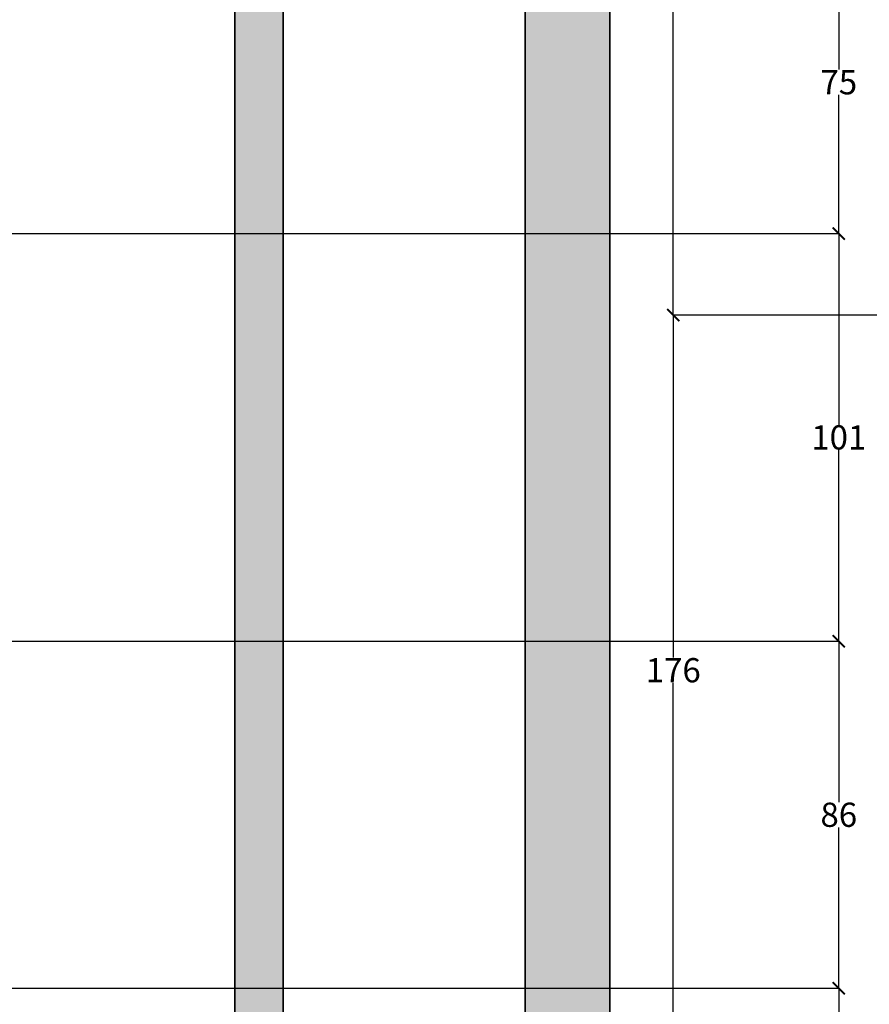
# Model space of a CAD drawing. Units: inches. Extents: x 925 to 2834, y 111 to 1355.
# Tile 12 of 25: x 1785 to 1996, y 638 to 882. Entities that reach past the tile are written whole.
import ezdxf

# ---------------------------------------------------------------- set-up
doc = ezdxf.new("R2010")
doc.units = ezdxf.units.IN
doc.header["$MEASUREMENT"] = 0
for name, color, linetype, lineweight in [('A-ANNO-DIMS', 2, 'Continuous', 18), ('A-ANNO-TTLB', 7, 'Continuous', 35), ('A-FLOR-PATT', 252, 'Continuous', 13)]:
    doc.layers.add(name, color=color, linetype=linetype, lineweight=lineweight)
doc.styles.get("Standard").update_dxf_attribs({"font": 'arial.ttf'})
doc.dimstyles.get("Standard").update_dxf_attribs({"dimtxt": 6, "dimasz": 3, "dimexe": 0.18, "dimexo": 0.0625, "dimgap": 0.09, "dimtad": 0, "dimtih": 1, "dimtoh": 1, "dimdec": 1, "dimzin": 0, "dimdsep": 46, "dimlunit": 3, "dimtxsty": 'Standard', "dimblk": 'ARCHTICK', "dimcen": 0.09, "dimadec": 0, "dimazin": 0, "dimtfac": 1, "dimtdec": 1, "dimtofl": 0, "dimtmove": 0, "dimatfit": 3, "dimfxl": 1, "dimtolj": 1, "dimtzin": 0, "dimarcsym": 0})

# ---------------------------------------------------------------- blocks, each defined once
blk = doc.blocks.new('_ArchTick')
at = {"color": 0, "linetype": 'ByBlock', "const_width": 0.15}
blk.add_lwpolyline([(-0.5, -0.5), (0.5, 0.5)], dxfattribs=at)
blk = doc.blocks.new('*D44')
at = {"layer": 'A-ANNO-DIMS', "color": 0, "lineweight": -2, "transparency": 16777216}
for p, q in [((1708.78, 641.59), (1988.62, 641.59)), ((1988.44, 641.59), (1988.44, 516.49)), ((1988.44, 385.09), (1988.44, 510.19)), ((1718.78, 385.09), (1988.62, 385.09))]:
    blk.add_line(p, q, dxfattribs=at)
at = {"layer": 'Defpoints', "color": 0, "transparency": 16777216}
for p in [(1708.71, 641.59), (1988.44, 641.59), (1718.71, 385.09)]:
    blk.add_point(p, dxfattribs=at)
at = {"layer": 'A-ANNO-DIMS', "color": 0, "lineweight": -2, "transparency": 16777216, "xscale": 3, "yscale": 3, "zscale": 3}
for p, rotation in [((1988.44, 641.59), 90), ((1988.44, 385.09), 270)]:
    blk.add_blockref('_ArchTick', p, dxfattribs=dict(at, rotation=rotation))
at = {"layer": 'A-ANNO-DIMS', "color": 0, "transparency": 16777216, "insert": (1988.44, 513.34), "char_height": 6, "attachment_point": 5}
blk.add_mtext('\\A1;256.5', dxfattribs=at)
blk = doc.blocks.new('*D45')
at = {"layer": 'A-ANNO-DIMS', "color": 0, "lineweight": -2, "transparency": 16777216}
for p, q in [((1708.78, 727.59), (1988.62, 727.59)), ((1988.44, 727.59), (1988.44, 687.74)), ((1988.44, 641.59), (1988.44, 681.44)), ((1708.78, 641.59), (1988.62, 641.59))]:
    blk.add_line(p, q, dxfattribs=at)
at = {"layer": 'Defpoints', "color": 0, "transparency": 16777216}
for p in [(1708.71, 727.59), (1988.44, 727.59), (1708.71, 641.59)]:
    blk.add_point(p, dxfattribs=at)
at = {"layer": 'A-ANNO-DIMS', "color": 0, "lineweight": -2, "transparency": 16777216, "xscale": 3, "yscale": 3, "zscale": 3}
for p, rotation in [((1988.44, 727.59), 90), ((1988.44, 641.59), 270)]:
    blk.add_blockref('_ArchTick', p, dxfattribs=dict(at, rotation=rotation))
at = {"layer": 'A-ANNO-DIMS', "color": 0, "transparency": 16777216, "insert": (1988.44, 684.59), "char_height": 6, "attachment_point": 5}
blk.add_mtext('\\A1;86', dxfattribs=at)
blk = doc.blocks.new('*D46')
at = {"layer": 'A-ANNO-DIMS', "color": 0, "lineweight": -2, "transparency": 16777216}
for p, q in [((1708.78, 828.59), (1988.62, 828.59)), ((1988.44, 828.59), (1988.44, 781.24)), ((1988.44, 727.59), (1988.44, 774.94)), ((1708.78, 727.59), (1988.62, 727.59))]:
    blk.add_line(p, q, dxfattribs=at)
at = {"layer": 'Defpoints', "color": 0, "transparency": 16777216}
for p in [(1708.71, 828.59), (1988.44, 828.59), (1708.71, 727.59)]:
    blk.add_point(p, dxfattribs=at)
at = {"layer": 'A-ANNO-DIMS', "color": 0, "lineweight": -2, "transparency": 16777216, "xscale": 3, "yscale": 3, "zscale": 3}
for p, rotation in [((1988.44, 828.59), 90), ((1988.44, 727.59), 270)]:
    blk.add_blockref('_ArchTick', p, dxfattribs=dict(at, rotation=rotation))
at = {"layer": 'A-ANNO-DIMS', "color": 0, "transparency": 16777216, "insert": (1988.44, 778.09), "char_height": 6, "attachment_point": 5}
blk.add_mtext('\\A1;101', dxfattribs=at)
blk = doc.blocks.new('*D47')
at = {"layer": 'A-ANNO-DIMS', "color": 0, "lineweight": -2, "transparency": 16777216}
for p, q in [((1708.78, 903.59), (1988.62, 903.59)), ((1988.44, 903.59), (1988.44, 869.23)), ((1988.44, 828.59), (1988.44, 862.95)), ((1708.78, 828.59), (1988.62, 828.59))]:
    blk.add_line(p, q, dxfattribs=at)
at = {"layer": 'Defpoints', "color": 0, "transparency": 16777216}
for p in [(1708.71, 903.59), (1988.44, 903.59), (1708.71, 828.59)]:
    blk.add_point(p, dxfattribs=at)
at = {"layer": 'A-ANNO-DIMS', "color": 0, "lineweight": -2, "transparency": 16777216, "xscale": 3, "yscale": 3, "zscale": 3}
for p, rotation in [((1988.44, 903.59), 90), ((1988.44, 828.59), 270)]:
    blk.add_blockref('_ArchTick', p, dxfattribs=dict(at, rotation=rotation))
at = {"layer": 'A-ANNO-DIMS', "color": 0, "transparency": 16777216, "insert": (1988.44, 866.09), "char_height": 6, "attachment_point": 5}
blk.add_mtext('\\A1;75', dxfattribs=at)
blk = doc.blocks.new('*D78')
at = {"layer": 'A-ANNO-DIMS', "color": 0, "lineweight": -2, "transparency": 16777216}
for p, q in [((2124.2, 808.4), (1947.23, 808.4)), ((1947.41, 808.4), (1947.41, 723.55)), ((1947.41, 632.4), (1947.41, 717.24)), ((2134.2, 632.4), (1947.23, 632.4))]:
    blk.add_line(p, q, dxfattribs=at)
at = {"layer": 'Defpoints', "color": 0, "transparency": 16777216}
for p in [(1947.41, 808.4), (2124.26, 808.4), (2134.26, 632.4)]:
    blk.add_point(p, dxfattribs=at)
at = {"layer": 'A-ANNO-DIMS', "color": 0, "lineweight": -2, "transparency": 16777216, "xscale": 3, "yscale": 3, "zscale": 3}
for p, rotation in [((1947.41, 808.4), 90), ((1947.41, 632.4), 270)]:
    blk.add_blockref('_ArchTick', p, dxfattribs=dict(at, rotation=rotation))
at = {"layer": 'A-ANNO-DIMS', "color": 0, "transparency": 16777216, "insert": (1947.41, 720.4), "char_height": 6, "attachment_point": 5}
blk.add_mtext('\\A1;176', dxfattribs=at)
blk = doc.blocks.new('*D79')
at = {"layer": 'A-ANNO-DIMS', "color": 0, "lineweight": -2, "transparency": 16777216}
for p, q in [((2143.61, 1057.4), (1947.23, 1057.4)), ((1947.41, 1057.4), (1947.41, 936.05)), ((1947.41, 808.4), (1947.41, 929.74)), ((2124.2, 808.4), (1947.23, 808.4))]:
    blk.add_line(p, q, dxfattribs=at)
at = {"layer": 'Defpoints', "color": 0, "transparency": 16777216}
for p in [(1947.41, 1057.4), (2143.68, 1057.4), (2124.26, 808.4)]:
    blk.add_point(p, dxfattribs=at)
at = {"layer": 'A-ANNO-DIMS', "color": 0, "lineweight": -2, "transparency": 16777216, "xscale": 3, "yscale": 3, "zscale": 3}
for p, rotation in [((1947.41, 1057.4), 90), ((1947.41, 808.4), 270)]:
    blk.add_blockref('_ArchTick', p, dxfattribs=dict(at, rotation=rotation))
at = {"layer": 'A-ANNO-DIMS', "color": 0, "transparency": 16777216, "insert": (1947.41, 932.9), "char_height": 6, "attachment_point": 5}
blk.add_mtext('\\A1;249', dxfattribs=at)

msp = doc.modelspace()

# ---------------------------------------------------------------- hatches: boundary and pattern name
at = {"layer": 'A-FLOR-PATT', "transparency": 33554605}
h = msp.add_hatch(color=256, dxfattribs=at)
h.dxf.hatch_style = 1
h.paths.add_polyline_path([(1931.688, 1294.5638), (991.7375, 1294.5638), (991.7375, 172.1134), (1931.688, 172.1134)])
h.paths.add_polyline_path([(1910.7128, 1273.5886), (1910.7128, 193.0886), (1012.7128, 193.0886), (1012.7128, 1273.5886)], flags=16)
h.paths.add_polyline_path([(1850.7128, 1213.5886), (1850.7128, 253.0886), (1072.7128, 253.0886), (1072.7128, 1213.5886)], flags=0)
h.paths.add_polyline_path([(1838.7128, 1201.5886), (1838.7128, 265.0886), (1084.7128, 265.0886), (1084.7128, 530.5886), (1084.7128, 1201.5886)], flags=0)
h.paths.add_polyline_path([(1547.6758, 1155.7396), (1547.6758, 1119.115), (1513.0687, 1119.115), (1513.0687, 1155.7396)], flags=0)
h.paths.add_polyline_path([(1600.1067, 1154.9439), (1634.7139, 1154.9439), (1634.7139, 1119.115), (1600.1067, 1119.115)], flags=0)
h.paths.add_polyline_path([(1505.2502, 1144.5358), (1505.2502, 1119.115), (1470.643, 1119.115), (1470.643, 1144.5358)], flags=0)
h.paths.add_polyline_path([(1559.1357, 1141.0962), (1593.7428, 1141.0962), (1593.7428, 1119.115), (1559.1357, 1119.115)], flags=0)
h.paths.add_polyline_path([(1462.8966, 1154.9439), (1462.8966, 1119.115), (1428.2895, 1119.115), (1428.2895, 1154.9439)], flags=0)
h.paths.add_polyline_path([(1642.4603, 1144.5358), (1677.0675, 1144.5358), (1677.0675, 1119.115), (1642.4603, 1119.115)], flags=0)
h.paths.add_polyline_path([(1422.3508, 1141.0962), (1422.3508, 1119.115), (1387.7436, 1119.115), (1387.7436, 1141.0962)], flags=0)
h.paths.add_polyline_path([(1684.8859, 1155.7396), (1719.4931, 1155.7396), (1719.4931, 1119.115), (1684.8859, 1119.115)], flags=0)
h.paths.add_polyline_path([(1718.7128, 1081.5886), (1718.7128, 1050.1249), (1715.7128, 1050.1249), (1715.7128, 1026.1249), (1715.7128, 1002.1249), (1718.7128, 1002.1249), (1730.7128, 1002.1249), (1730.7128, 998.1249), (1730.7128, 990.1249), (1730.7128, 986.1249), (1718.7128, 986.1249), (1718.7128, 893.5886), (1715.3735, 893.5886), (1715.3735, 891.5886), (1713.3735, 891.5886, 0.41421356), (1677.3735, 855.5886), (1713.3735, 855.5886), (1713.3735, 853.5886), (1715.3735, 853.5886), (1715.3735, 851.5886), (1718.7128, 851.5886), (1718.7128, 821.5865), (1734.4655, 821.5865), (1734.3735, 819.5886, -0.41421356), (1712.4415, 793.5886), (1712.4415, 791.5886), (1718.7128, 791.5886), (1718.7128, 717.5886), (1718.7128, 669.5886), (1732.7128, 669.5886), (1732.7128, 665.5886), (1732.7128, 641.5886), (1732.7128, 634.5886), (1732.7128, 610.5886), (1732.7128, 603.5886), (1718.7128, 603.5886), (1718.7128, 385.0886), (1434.2128, 385.0886), (1434.2128, 530.5886), (1410.2128, 530.5886), (1408.2128, 530.5886), (1408.2128, 532.5886, 0.41421356), (1372.2128, 568.5886), (1372.2128, 532.5886), (1370.2128, 532.5886), (1370.2128, 530.5886), (1368.2128, 530.5886), (1282.2128, 530.5886), (1210.2128, 530.5886), (1200.2128, 530.5886), (1200.2128, 542.1915), (1183.2307, 542.1915), (1183.2307, 546.1915), (1200.2128, 546.1915), (1200.2128, 572.1915), (1183.2307, 572.1915), (1183.2307, 576.1915), (1200.2128, 576.1915), (1200.2128, 727.5886), (1210.2128, 727.5886), (1234.2128, 727.5886), (1259.7128, 727.5886), (1259.7128, 775.5886), (1259.7128, 799.5886), (1259.7128, 847.5886), (1259.7128, 993.5872), (1259.7128, 1065.5872), (1259.7128, 1071.5886), (1219.6318, 1071.5886), (1219.6318, 1081.5886), (1084.7128, 1081.5886), (1084.7128, 1119.115), (1256.8974, 1119.115), (1256.8974, 1154.9439), (1291.5046, 1154.9439), (1291.5046, 1119.115), (1256.8974, 1119.115), (1256.6723, 1081.5886), (1293.7128, 1081.5886), (1341.7128, 1081.5886), (1341.7128, 1093.5886), (1347.7128, 1093.5886), (1371.7128, 1093.5886), (1377.7128, 1093.5886), (1377.7128, 1081.5886), (1668.7128, 1081.5886), (1668.7128, 1117.5886), (1675.7128, 1117.5886), (1711.7128, 1117.5886), (1718.7128, 1117.5886)], flags=0)
h.paths.add_polyline_path([(1376.2838, 1155.7396), (1376.2838, 1119.115), (1341.6766, 1119.115), (1341.6766, 1155.7396)], flags=0)
h.paths.add_polyline_path([(1341.7128, 1076.0886), (1293.7128, 1076.0886), (1293.7128, 1071.5886), (1269.7128, 1071.5886), (1269.7128, 1065.5872), (1266.7128, 1065.5872), (1266.7128, 1029.5872), (1265.7128, 1029.5872), (1265.7128, 993.5872), (1269.7128, 993.5872), (1269.7128, 903.5886), (1269.7128, 893.5886), (1269.7128, 847.5886), (1265.2128, 847.5886), (1265.2128, 799.5886), (1269.7128, 799.5886), (1269.7128, 775.5886), (1265.2128, 775.5886), (1265.2128, 727.5886), (1269.7128, 727.5886), (1444.2128, 727.5886), (1444.2128, 717.5886), (1234.2128, 717.5886), (1234.2128, 722.0886), (1210.2128, 722.0886), (1210.2128, 717.5886), (1210.2128, 540.5886), (1210.2128, 536.0886), (1282.2128, 536.0886), (1282.2128, 535.0886), (1210.2128, 535.0886), (1210.2128, 540.5886), (1210.2128, 717.5886), (1210.2128, 723.0886), (1234.2128, 723.0886), (1234.2128, 717.5886), (1444.2128, 717.5886), (1444.2128, 727.5886), (1269.7128, 727.5886), (1264.2128, 727.5886), (1264.2128, 775.5886), (1269.7128, 775.5886), (1269.7128, 799.5886), (1264.2128, 799.5886), (1264.2128, 847.5886), (1269.7128, 847.5886), (1269.7128, 893.5886), (1269.7128, 903.5886), (1269.7128, 993.5872), (1264.7128, 993.5872), (1264.7128, 1029.5872), (1265.7128, 1029.5872), (1265.7128, 1065.5872), (1269.7128, 1065.5872), (1269.7128, 1071.5886), (1293.7128, 1071.5886), (1293.7128, 1077.0886), (1341.7128, 1077.0886)], flags=0)
h.paths.add_polyline_path([(1730.9529, 1141.0962), (1765.5601, 1141.0962), (1765.5601, 1119.115), (1730.9529, 1119.115)], flags=0)
h.paths.add_polyline_path([(1333.8582, 1144.5358), (1333.8582, 1119.115), (1299.251, 1119.115), (1299.251, 1144.5358)], flags=0)
h.paths.add_polyline_path([(1592.7128, 968.5886), (1596.0342, 968.5886), (1602.7128, 968.5886), (1708.7128, 968.5886), (1708.7128, 903.5886), (1602.7128, 903.5886), (1602.7128, 938.5886), (1592.7128, 938.5886), (1592.7128, 903.5886), (1451.7128, 903.5886), (1451.7128, 893.5886), (1511.7128, 893.5886), (1511.7128, 881.5886), (1515.2128, 881.5886), (1518.7128, 881.5886), (1518.7128, 893.5886), (1592.7128, 893.5886), (1592.7128, 799.5886), (1518.7128, 799.5886), (1518.7128, 857.5886), (1511.7128, 857.5886), (1511.7128, 799.5886), (1511.7128, 772.0886), (1521.7128, 772.0886), (1521.7128, 792.5886), (1592.7128, 792.5886), (1592.7128, 727.5886), (1521.7128, 727.5886), (1521.7128, 748.0886), (1511.7128, 748.0886), (1511.7128, 717.5886), (1708.7128, 717.5886), (1714.2128, 717.5886), (1714.2128, 669.5886), (1708.7128, 669.5886), (1708.7128, 641.5886), (1492.2128, 641.5886), (1492.2128, 631.5886), (1621.2128, 631.5886), (1621.2128, 443.0886), (1625.7128, 443.0886), (1625.7128, 503.0886), (1625.7128, 507.5886), (1625.7128, 631.5886), (1708.7128, 631.5886), (1708.7128, 507.5886), (1655.7128, 507.5886), (1655.7128, 503.0886), (1708.7128, 503.0886), (1708.7128, 395.0886), (1625.7128, 395.0886), (1625.7128, 419.0886), (1621.2128, 419.0886), (1621.2128, 395.0886), (1482.2128, 395.0886), (1482.2128, 385.0886), (1434.2128, 385.0886), (1434.2128, 433.0886), (1444.2128, 433.0886), (1444.2128, 631.5886), (1450.2128, 631.5886), (1450.2128, 634.91), (1452.2128, 634.91), (1452.2128, 669.5886), (1454.2128, 669.5886, -0.40021217), (1490.1712, 635.3173), (1492.2128, 635.3173), (1492.2128, 641.5886), (1564.7128, 641.5886), (1564.7128, 677.5886), (1672.7128, 677.5886), (1672.7128, 681.5886), (1564.7128, 681.5886), (1564.7128, 717.5886), (1511.7128, 717.5886), (1511.7128, 748.0886), (1511.7128, 772.0886), (1511.7128, 799.5886), (1511.7128, 857.5886), (1511.8913, 857.5886), (1511.8913, 859.5886), (1515.6201, 859.5886, 0.41421356), (1537.552, 879.5886), (1513.552, 879.5886), (1511.8913, 879.5886), (1511.8913, 881.5886), (1511.7128, 881.5886), (1511.7128, 893.5886), (1451.7128, 893.5886), (1451.7128, 903.5886), (1592.7128, 903.5886), (1592.7128, 938.5886), (1592.7128, 940.5886), (1596.4415, 940.5886, 0.41421356), (1618.3735, 966.5886), (1594.3735, 966.5886), (1592.7128, 966.5886)], flags=0)
h.paths.add_polyline_path([(1377.7128, 903.5886), (1377.7128, 893.5886), (1305.7128, 893.5886), (1305.7128, 903.5886)], flags=0)
h.paths.add_polyline_path([(1708.7128, 821.5886), (1712.0342, 821.5886), (1712.0342, 819.5886), (1710.3735, 819.5886), (1708.7128, 819.5886)], flags=0)
h.paths.add_polyline_path([(1576.7128, 695.1992), (1575.5896, 693.6649), (1575.9687, 694.6994), (1575.4438, 695.1992), (1575.9687, 695.699), (1575.5896, 696.7335)], flags=0)
h.paths.add_polyline_path([(1565.9817, 662.3134), (1565.4568, 661.8136), (1565.8359, 660.7791), (1564.7128, 662.3134), (1565.8359, 663.8477), (1565.4568, 662.8132)], flags=0)
h.paths.add_polyline_path([(1444.2128, 433.0886), (1444.2128, 395.0886), (1482.2128, 395.0886), (1482.2128, 389.0886), (1438.2128, 389.0886), (1438.2128, 391.8608), (1438.2128, 433.0886)], flags=0)
h.paths.add_polyline_path([(1410.2128, 506.5886), (1410.2128, 289.0886), (1108.7128, 289.0886), (1108.7128, 506.5886)], flags=0)
h.paths.add_polyline_path([(1612.3153, 838.3016), (1680.4151, 838.3016), (1680.4151, 851.3131), (1612.3153, 851.3131)], flags=8)
h.paths.add_polyline_path([(1208.3174, 395.0436), (1282.1017, 395.0436), (1282.1017, 408.0552), (1208.3174, 408.0552)], flags=8)
h.paths.add_polyline_path([(1291.8049, 598.7427), (1369.8017, 598.7427), (1369.8017, 611.7542), (1291.8049, 611.7542)], flags=8)
h.paths.add_polyline_path([(1119.679, 917.3022), (1191.0817, 917.3022), (1191.0817, 930.3137), (1119.679, 930.3137)], flags=8)
h.paths.add_polyline_path([(1332.2261, 815.9808), (1410.2258, 815.9808), (1410.2258, 829.001), (1332.2261, 829.001)], flags=8)
h.paths.add_polyline_path([(1390.9013, 955.8158), (1475.4981, 955.8158), (1475.4981, 968.8273), (1390.9013, 968.8273)], flags=8)
h.paths.add_polyline_path([(1620.3436, 998.9325), (1688.4434, 998.9325), (1688.4434, 1011.944), (1620.3436, 1011.944)], flags=8)
h.paths.add_polyline_path([(1620.3436, 914.1039), (1691.7405, 914.1039), (1691.7405, 927.1155), (1620.3436, 927.1155)], flags=8)
h.paths.add_polyline_path([(1521.4542, 816.005), (1589.5569, 816.005), (1589.5569, 829.0253), (1521.4542, 829.0253)], flags=8)
h.paths.add_polyline_path([(1528.524, 740.3497), (1602.3082, 740.3497), (1602.3082, 753.3613), (1528.524, 753.3613)], flags=8)
h.paths.add_polyline_path([(1627.6094, 762.6128), (1702.3091, 762.6128), (1702.3091, 775.6244), (1627.6094, 775.6244)], flags=8)
h.paths.add_polyline_path([(1610.5442, 657.2751), (1684.3284, 657.2751), (1684.3284, 670.2867), (1610.5442, 670.2867)], flags=8)
h.paths.add_polyline_path([(1636.6983, 519.472), (1711.3981, 519.472), (1711.3981, 532.4835), (1636.6983, 532.4835)], flags=8)
h.paths.add_polyline_path([(1616.8577, 424.8539), (1694.8545, 424.8539), (1694.8545, 437.8654), (1616.8577, 437.8654)], flags=8)
h.paths.add_polyline_path([(1506.1456, 460.8838), (1579.9299, 460.8838), (1579.9299, 473.8953), (1506.1456, 473.8953)], flags=8)
h.paths.add_polyline_path([(1624.6119, 784.6011), (1696.9185, 784.6011), (1696.9185, 797.7864), (1624.6119, 797.7864)], flags=8)
h.paths.add_polyline_path([(1606.3732, 854.2194), (1683.3039, 854.2194), (1683.3039, 867.4048), (1606.3732, 867.4048)], flags=8)
h.paths.add_polyline_path([(1127.8008, 940.3581), (1165.1637, 940.3581), (1165.1637, 953.5348), (1127.8008, 953.5348)], flags=8)
h.paths.add_polyline_path([(1620.8657, 1019.4968), (1677.3447, 1019.4968), (1677.3447, 1032.6735), (1620.8657, 1032.6735)], flags=8)
h.paths.add_polyline_path([(1620.8643, 930.1821), (1703.0564, 930.1821), (1703.0564, 943.3675), (1620.8643, 943.3675)], flags=8)
h.paths.add_polyline_path([(1324.5702, 836.8338), (1408.0892, 836.8338), (1408.0892, 850.0191), (1324.5702, 850.0191)], flags=8)
h.paths.add_polyline_path([(1281.6584, 622.8885), (1383.6213, 622.8885), (1383.6213, 636.0739), (1281.6584, 636.0739)], flags=8)
h.paths.add_polyline_path([(1210.6721, 416.7893), (1269.1299, 416.7893), (1269.1299, 429.9747), (1210.6721, 429.9747)], flags=8)
h.paths.add_polyline_path([(1507.8264, 477.4836), (1586.7329, 477.4836), (1586.7329, 490.669), (1507.8264, 490.669)], flags=8)
h.paths.add_polyline_path([(1643.6238, 443.8135), (1696.6696, 443.8135), (1696.6696, 456.5643), (1643.6238, 456.5643)], flags=8)
h.paths.add_polyline_path([(1647.2466, 540.5638), (1693.1825, 540.5638), (1693.1825, 553.7491), (1647.2466, 553.7491)], flags=8)
h.paths.add_polyline_path([(1626.0633, 668.5064), (1673.3174, 668.5064), (1673.3174, 681.6831), (1626.0633, 681.6831)], flags=8)
h.paths.add_polyline_path([(1538.2915, 830.7872), (1567.5942, 830.7872), (1567.5942, 843.5293), (1538.2915, 843.5293)], flags=8)
h.paths.add_polyline_path([(1530.9338, 754.0477), (1559.576, 754.0477), (1559.576, 766.7898), (1530.9338, 766.7898)], flags=8)
h.paths.add_polyline_path([(1351.2461, 979.2309), (1513.8919, 979.2309), (1513.8919, 992.4076), (1351.2461, 992.4076)], flags=8)
at = {"layer": 'A-FLOR-PATT'}
h = msp.add_hatch(color=256, dxfattribs=at)
h.dxf.hatch_style = 1
h.paths.add_polyline_path([(1850.7128, 1213.5886), (1072.7128, 1213.5886), (1072.7128, 253.0886), (1850.7128, 253.0886)])
h.paths.add_polyline_path([(1084.7128, 1201.5886), (1838.7128, 1201.5886), (1838.7128, 265.0886), (1084.7128, 265.0886)], flags=16)
h.paths.add_polyline_path([(1183.2307, 576.1915), (1200.2128, 576.1915), (1200.2128, 727.5886), (1210.2128, 727.5886), (1234.2128, 727.5886), (1259.7128, 727.5886), (1259.7128, 775.5886), (1259.7128, 799.5886), (1259.7128, 847.5886), (1259.7128, 993.5872), (1259.7128, 1065.5872), (1259.7128, 1071.5886), (1219.6318, 1071.5886), (1219.6318, 1081.5886), (1293.7128, 1081.5886), (1341.7128, 1081.5886), (1341.7128, 1093.5886), (1347.7128, 1093.5886), (1347.7128, 1081.5886), (1371.7128, 1081.5886), (1371.7128, 1093.5886), (1377.7128, 1093.5886), (1377.7128, 1081.5886), (1668.7128, 1081.5886), (1668.7128, 1117.5886), (1675.7128, 1117.5886), (1675.7128, 1081.5886), (1711.7128, 1081.5886), (1711.7128, 1117.5886), (1718.7128, 1117.5886), (1718.7128, 1081.5886), (1718.7128, 1050.1249), (1715.7128, 1050.1249), (1715.7128, 1026.1249), (1715.7128, 1002.1249), (1718.7128, 1002.1249), (1730.7128, 1002.1249), (1730.7128, 998.1249), (1730.7128, 990.1249), (1730.7128, 986.1249), (1718.7128, 986.1249), (1718.7128, 893.5886), (1715.3735, 893.5886), (1715.3735, 891.5886), (1713.3735, 891.5886, 0.41421356), (1677.3735, 855.5886), (1713.3735, 855.5886), (1713.3735, 853.5886), (1715.3735, 853.5886), (1715.3735, 851.5886), (1718.7128, 851.5886), (1718.7128, 821.5865), (1734.4655, 821.5865), (1734.3735, 819.5886, -0.41421356), (1712.4415, 793.5886), (1712.4415, 791.5886), (1718.7128, 791.5886), (1718.7128, 717.5886), (1718.7128, 669.5886), (1732.7128, 669.5886), (1732.7128, 665.5886), (1732.7128, 641.5886), (1732.7128, 634.5886), (1732.7128, 610.5886), (1732.7128, 603.5886), (1718.7128, 603.5886), (1718.7128, 385.0886), (1434.2128, 385.0886), (1434.2128, 433.0886), (1434.2128, 530.5886), (1410.2128, 530.5886), (1408.2128, 530.5886), (1408.2128, 532.5886, 0.41421356), (1372.2128, 568.5886), (1372.2128, 532.5886), (1370.2128, 532.5886), (1370.2128, 530.5886), (1368.2128, 530.5886), (1282.2128, 530.5886), (1210.2128, 530.5886), (1200.2128, 530.5886), (1200.2128, 542.1915), (1183.2307, 542.1915), (1183.2307, 546.1915), (1200.2128, 546.1915), (1200.2128, 572.1915), (1183.2307, 572.1915)], flags=0)
h.paths.add_polyline_path([(1210.2128, 717.5886), (1210.2128, 723.0886), (1234.2128, 723.0886), (1234.2128, 717.5886), (1444.2128, 717.5886), (1444.2128, 727.5886), (1269.7128, 727.5886), (1264.2128, 727.5886), (1264.2128, 775.5886), (1269.7128, 775.5886), (1269.7128, 799.5886), (1264.2128, 799.5886), (1264.2128, 847.5886), (1269.7128, 847.5886), (1269.7128, 893.5886), (1269.7128, 903.5886), (1269.7128, 993.5872), (1264.7128, 993.5872), (1264.7128, 1029.5872), (1265.7128, 1029.5872), (1265.7128, 1065.5872), (1269.7128, 1065.5872), (1269.7128, 1071.5886), (1293.7128, 1071.5886), (1293.7128, 1077.0886), (1341.7128, 1077.0886), (1341.7128, 1076.0886), (1293.7128, 1076.0886), (1293.7128, 1071.5886), (1269.7128, 1071.5886), (1269.7128, 1065.5872), (1266.7128, 1065.5872), (1266.7128, 1029.5872), (1265.7128, 1029.5872), (1265.7128, 993.5872), (1269.7128, 993.5872), (1269.7128, 903.5886), (1269.7128, 893.5886), (1269.7128, 847.5886), (1265.2128, 847.5886), (1265.2128, 799.5886), (1269.7128, 799.5886), (1269.7128, 775.5886), (1265.2128, 775.5886), (1265.2128, 727.5886), (1269.7128, 727.5886), (1444.2128, 727.5886), (1444.2128, 717.5886), (1234.2128, 717.5886), (1234.2128, 722.0886), (1210.2128, 722.0886), (1210.2128, 717.5886), (1210.2128, 540.5886), (1210.2128, 536.0886), (1282.2128, 536.0886), (1282.2128, 535.0886), (1210.2128, 535.0886), (1210.2128, 540.5886)], flags=0)
h.paths.add_polyline_path([(1450.2128, 634.91), (1452.2128, 634.91), (1452.2128, 669.5886), (1454.2128, 669.5886, -0.40021217), (1490.1712, 635.3173), (1492.2128, 635.3173), (1492.2128, 641.5886), (1564.7128, 641.5886), (1564.7128, 677.5886), (1672.7128, 677.5886), (1672.7128, 681.5886), (1564.7128, 681.5886), (1564.7128, 717.5886), (1511.7128, 717.5886), (1511.7128, 748.0886), (1511.7128, 772.0886), (1511.7128, 799.5886), (1511.7128, 857.5886), (1511.8913, 857.5886), (1511.8913, 859.5886), (1515.6201, 859.5886, 0.41421356), (1537.552, 879.5886), (1513.552, 879.5886), (1511.8913, 879.5886), (1511.8913, 881.5886), (1511.7128, 881.5886), (1511.7128, 893.5886), (1451.7128, 893.5886), (1451.7128, 903.5886), (1592.7128, 903.5886), (1592.7128, 938.5886), (1592.7128, 940.5886), (1596.4415, 940.5886, 0.41421356), (1618.3735, 966.5886), (1594.3735, 966.5886), (1592.7128, 966.5886), (1592.7128, 968.5886), (1596.0342, 968.5886), (1602.7128, 968.5886), (1708.7128, 968.5886), (1708.7128, 903.5886), (1602.7128, 903.5886), (1602.7128, 938.5886), (1592.7128, 938.5886), (1592.7128, 903.5886), (1451.7128, 903.5886), (1451.7128, 893.5886), (1511.7128, 893.5886), (1511.7128, 881.5886), (1518.7128, 881.5886), (1518.7128, 893.5886), (1592.7128, 893.5886), (1592.7128, 799.5886), (1518.7128, 799.5886), (1518.7128, 857.5886), (1511.7128, 857.5886), (1511.7128, 799.5886), (1511.7128, 772.0886), (1521.7128, 772.0886), (1521.7128, 792.5886), (1592.7128, 792.5886), (1592.7128, 727.5886), (1521.7128, 727.5886), (1521.7128, 748.0886), (1511.7128, 748.0886), (1511.7128, 717.5886), (1708.7128, 717.5886), (1714.2128, 717.5886), (1714.2128, 669.5886), (1708.7128, 669.5886), (1708.7128, 641.5886), (1492.2128, 641.5886), (1492.2128, 631.5886), (1621.2128, 631.5886), (1621.2128, 443.0886), (1625.7128, 443.0886), (1625.7128, 503.0886), (1625.7128, 507.5886), (1625.7128, 631.5886), (1708.7128, 631.5886), (1708.7128, 507.5886), (1655.7128, 507.5886), (1655.7128, 503.0886), (1708.7128, 503.0886), (1708.7128, 395.0886), (1625.7128, 395.0886), (1625.7128, 419.0886), (1621.2128, 419.0886), (1621.2128, 395.0886), (1482.2128, 395.0886), (1482.2128, 389.0886), (1438.2128, 389.0886), (1438.2128, 391.8608), (1438.2128, 433.0886), (1444.2128, 433.0886), (1444.2128, 631.5886), (1450.2128, 631.5886)], flags=0)
h.paths.add_polyline_path([(1444.2128, 433.0886), (1444.2128, 395.0886), (1482.2128, 395.0886), (1482.2128, 391.0886), (1440.2128, 391.0886), (1440.2128, 391.8608), (1440.2128, 433.0886)], flags=0)
h.paths.add_polyline_path([(1305.7128, 893.5886), (1305.7128, 903.5886), (1377.7128, 903.5886), (1377.7128, 893.5886)], flags=0)
h.paths.add_polyline_path([(1564.7128, 662.3134), (1565.8359, 663.8477), (1565.4568, 662.8132), (1565.9817, 662.3134), (1565.4568, 661.8136), (1565.8359, 660.7791)], flags=0)
h.paths.add_polyline_path([(1575.4438, 695.1992), (1575.9687, 695.699), (1575.5896, 696.7335), (1576.7128, 695.1992), (1575.5896, 693.6649), (1575.9687, 694.6994)], flags=0)
h.paths.add_polyline_path([(1708.7128, 821.5886), (1712.0342, 821.5886), (1712.0342, 819.5886), (1710.3735, 819.5886), (1708.7128, 819.5886)], flags=0)

# ---------------------------------------------------------------- linework, layer by layer
at = {"layer": 'A-ANNO-TTLB'}
for p, q in [((1838.7128, 1201.5886), (1838.7128, 265.0886)), ((1838.7128, 265.0886), (1838.7128, 1081.5886))]:
    msp.add_line(p, q, dxfattribs=at)
for points in [[(991.7375, 172.1134), (1931.688, 172.1134), (1931.688, 1294.5638), (991.7375, 1294.5638)], [(1012.7128, 193.0886), (1910.7128, 193.0886), (1910.7128, 1273.5886), (1012.7128, 1273.5886)], [(1072.7128, 253.0886), (1850.7128, 253.0886), (1850.7128, 1213.5886), (1072.7128, 1213.5886)], [(1084.7128, 265.0886), (1838.7128, 265.0886), (1838.7128, 1201.5886), (1084.7128, 1201.5886)]]:
    msp.add_lwpolyline(points, close=True, dxfattribs=at)

# ---------------------------------------------------------------- dimensions: what is measured, and where the dimension line sits
at = {"layer": 'A-ANNO-DIMS'}
for base, p1, p2, override, picture, middle in [((1947.408, 1057.3964), (2124.258, 808.3964), (2143.677, 1057.3964), {"dimdec": 0, "dimlfac": 1, "dimrnd": 0, "dimzin": 0, "dimdsep": 46, "dimlunit": 2}, '*D79', (1947.408, 932.8964)), ((1988.438, 903.5886), (1708.7128, 828.5886), (1708.7128, 903.5886), {"dimdec": 0, "dimlfac": 1, "dimrnd": 0, "dimzin": 0, "dimdsep": 46, "dimlunit": 2}, '*D47', (1988.438, 866.0886)), ((1988.438, 828.5886), (1708.7128, 727.5886), (1708.7128, 828.5886), {"dimdec": 0, "dimlfac": 1, "dimrnd": 0, "dimzin": 0, "dimdsep": 46, "dimlunit": 2}, '*D46', (1988.438, 778.0886)), ((1947.408, 808.3964), (2134.258, 632.3964), (2124.258, 808.3964), {"dimdec": 0, "dimlfac": 1, "dimrnd": 0, "dimzin": 0, "dimdsep": 46, "dimlunit": 2}, '*D78', (1947.408, 720.3964)), ((1988.438, 727.5886), (1708.7128, 641.5886), (1708.7128, 727.5886), {"dimdec": 0, "dimlfac": 1, "dimrnd": 0, "dimzin": 0, "dimdsep": 46, "dimlunit": 2}, '*D45', (1988.438, 684.5886)), ((1988.438, 641.5886), (1718.7128, 385.0886), (1708.7128, 641.5886), {"dimdec": 1, "dimlfac": 1, "dimrnd": 0, "dimzin": 0, "dimdsep": 46, "dimlunit": 2}, '*D44', (1988.438, 513.3386))]:
    dim = msp.add_linear_dim(base=base, p1=p1, p2=p2, angle=90, dimstyle='Standard', override=override, dxfattribs=at)
    dim.commit()
    dim.dimension.update_dxf_attribs({"geometry": picture, "text_midpoint": middle})

doc.saveas('drawing.dxf')
